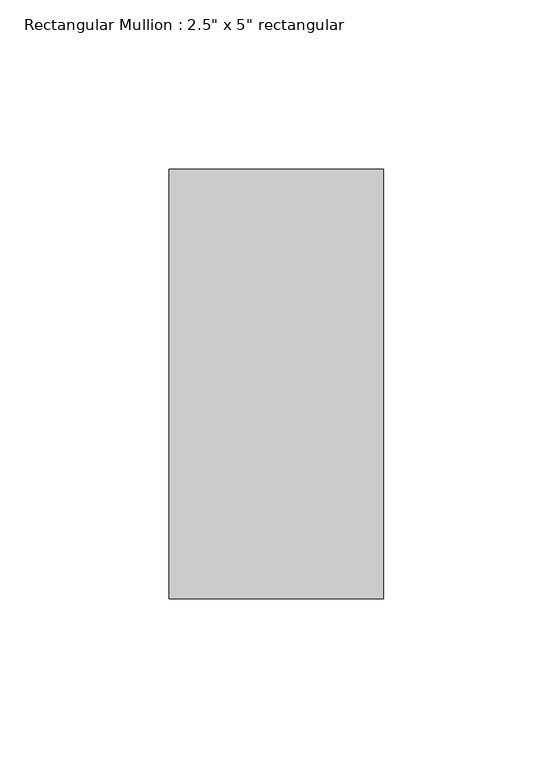
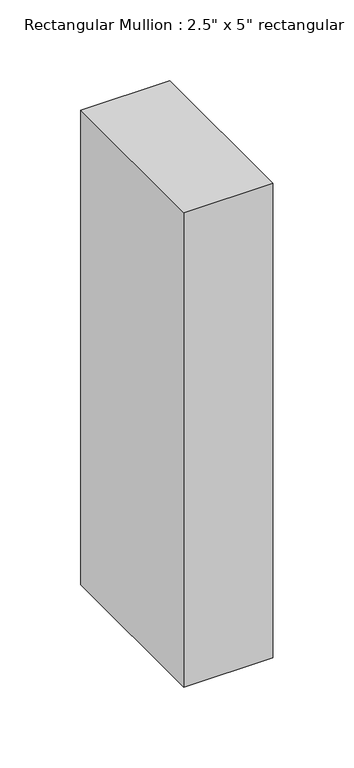
"""IFC4 building model written with IfcOpenShell, lengths in millimetres: member geometry."""

from ifc_helpers import new_model, si_unit, frame, origin, place, context, project, spatial, polyline, outline, extrude, source, transform, mapped, element, save


def member_76ec7c80(model_context):
    return source(origin(), model_context, "Body", "SweptSolid", [
        extrude(outline(polyline([(0.0, 63.5), (0.0, -63.5), (-63.5, -63.5), (-63.5, 63.5), (0.0, 63.5)])), frame((0.0, 0.0, -357.7166667), z_axis=(0.0, 0.0, 1.0), x_axis=(1.0, 0.0, 0.0)), (0.0, 0.0, 1.0), 357.7166667),
    ])


if __name__ == "__main__":
    model = new_model("IFC4")
    model_context = context("Model", 3, world=origin())
    ifc_project = project(units=[si_unit("LENGTHUNIT", "METRE", prefix="MILLI")], contexts=[model_context])
    site = spatial("IfcSite", under=ifc_project)
    building = spatial("IfcBuilding", under=site)
    placement = place(None, origin())
    member_shape = member_76ec7c80(model_context)
    element("IfcMember", 1, ObjectType="Rectangular Mullion : 2.5\" x 5\" rectangular", at=placement, inside=building, context=model_context, shape_type="MappedRepresentation", body=[
        mapped(member_shape, transform((0.0, 0.0, 0.0), x_axis=(1.0, 0.0, 0.0), y_axis=(0.0, 1.0, 0.0), z_axis=(0.0, 0.0, 1.0))),
    ])
    save(model, "model.ifc")

# Revit data of these elements
# Type "Rectangular Mullion : 2.5\" x 5\" rectangular"
#   built-in parameter 1007304 = 0.416667 (stored number, unit not read)
#   built-in parameter 1007301 = 0.104167 (stored number, unit not read)
#   built-in parameter 1007300 = 0.104167 (stored number, unit not read)
# Element 1 (IfcMember, "Rectangular Mullion : 2.5\" x 5\" rectangular")
#   Materials on its faces: "Aluminum"
# Materials
#   "Aluminum": class "Metal", colour RGB 247 247 247, transparency 0, Description = "Aluminum 6061", Cost = 0
